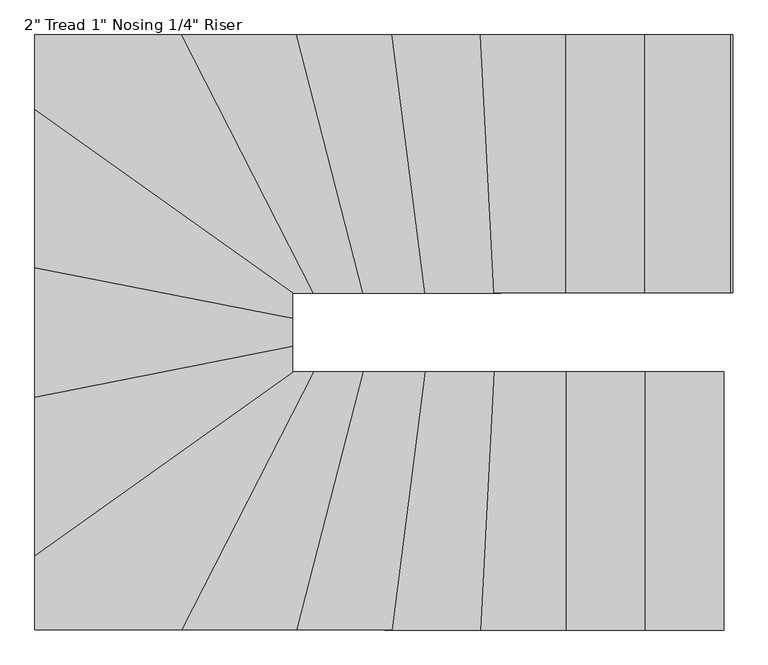
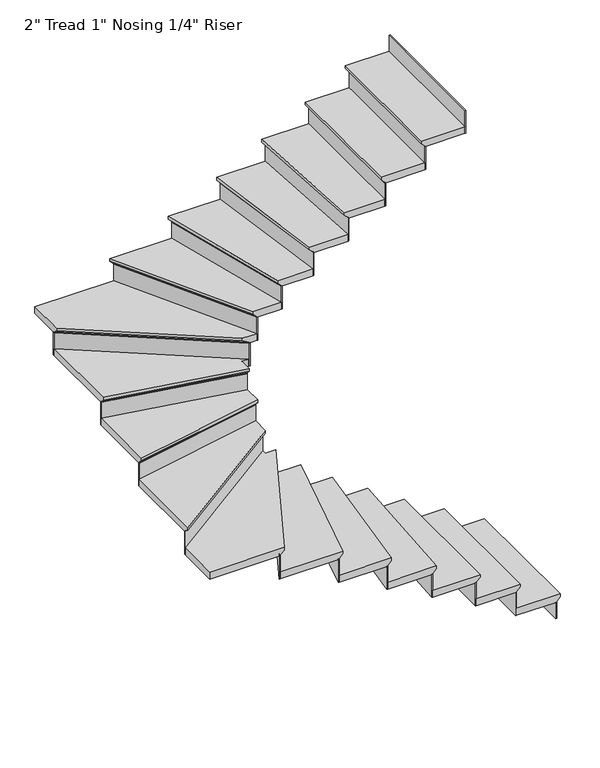
"""IFC4 building model written with IfcOpenShell, lengths in millimetres: stair flight geometry."""

from ifc_helpers import new_model, si_unit, origin, place, context, project, spatial, faceted_brep, source, transform, mapped, element, save


def stair_flight_5420025d(model_context):
    return source(origin(), model_context, "Body", "Brep", [
        faceted_brep([(-1761.7449167, -345.7070853, 3350.6833333), (-1761.7449167, -345.7070853, 3369.7333333), (-1761.7449167, -1260.1070853, 3369.7333333), (-1761.7449167, -1260.1070853, 3350.6833333), (-1787.1449167, -345.7070853, 3325.2833333), (-1787.1449167, -1260.1070853, 3325.2833333), (-2066.5449167, -345.7070853, 3369.7333333), (-2066.5449167, -1260.1070853, 3369.7333333), (-1787.1449167, -1260.1070853, 3318.9333333), (-2066.5449167, -1260.1070853, 3318.9333333), (-2066.5449167, -345.7070853, 3318.9333333), (-1787.1449167, -345.7070853, 3318.9333333)], [[[0, 1, 2, 3]], [[4, 0, 3, 5]], [[2, 1, 6, 7]], [[8, 9, 10, 11]], [[2, 7, 9, 8, 5, 3]], [[8, 11, 4, 5]], [[6, 1, 0, 4, 11, 10]], [[7, 6, 10, 9]]]),
        faceted_brep([(-1787.1449167, -345.7070853, 3318.9333333), (-1787.1449167, -345.7070853, 3200.4), (-1793.4949167, -345.7070853, 3200.4), (-1793.4949167, -345.7070853, 3318.9333333), (-1787.1449167, -1260.1070853, 3318.9333333), (-1793.4949167, -1260.1070853, 3318.9333333), (-1793.4949167, -1260.1070853, 3200.4), (-1787.1449167, -1260.1070853, 3200.4)], [[[0, 1, 2, 3]], [[4, 5, 6, 7]], [[1, 0, 4, 7]], [[2, 1, 7, 6]], [[3, 2, 6, 5]], [[0, 3, 5, 4]]]),
        faceted_brep([(-2066.5449167, -345.7070853, 3488.2666667), (-2066.5449167, -345.7070853, 3318.9333333), (-2072.8949167, -345.7070853, 3318.9333333), (-2072.8949167, -345.7070853, 3488.2666667), (-2066.5449167, -1260.1070853, 3488.2666667), (-2072.8949167, -1260.1070853, 3488.2666667), (-2072.8949167, -1260.1070853, 3318.9333333), (-2066.5449167, -1260.1070853, 3318.9333333)], [[[0, 1, 2, 3]], [[4, 5, 6, 7]], [[1, 0, 4, 7]], [[2, 1, 7, 6]], [[3, 2, 6, 5]], [[0, 3, 5, 4]]]),
        faceted_brep([(-2041.1449167, -1260.1070853, 3539.0666667), (-2041.1449167, -345.7070853, 3539.0666667), (-2345.9449167, -345.7070853, 3539.0666667), (-2345.9449167, -1260.1070853, 3539.0666667), (-2066.5449167, -1260.1070853, 3488.2666667), (-2345.9449167, -1260.1070853, 3488.2666667), (-2345.9449167, -345.7070853, 3488.2666667), (-2066.5449167, -345.7070853, 3488.2666667), (-2066.5449167, -1260.1070853, 3494.6166667), (-2041.1449167, -1260.1070853, 3520.0166667), (-2066.5449167, -345.7070853, 3494.6166667), (-2041.1449167, -345.7070853, 3520.0166667)], [[[0, 1, 2, 3]], [[4, 5, 6, 7]], [[0, 3, 5, 4, 8, 9]], [[4, 7, 10, 8]], [[2, 1, 11, 10, 7, 6]], [[3, 2, 6, 5]], [[11, 1, 0, 9]], [[10, 11, 9, 8]]]),
        faceted_brep([(-2345.9449167, -345.7070853, 3657.6), (-2345.9449167, -345.7070853, 3488.2666667), (-2352.2949167, -345.7070853, 3488.2666667), (-2352.2949167, -345.7070853, 3657.6), (-2345.9449167, -1260.1070853, 3657.6), (-2352.2949167, -1260.1070853, 3657.6), (-2352.2949167, -1260.1070853, 3488.2666667), (-2345.9449167, -1260.1070853, 3488.2666667)], [[[0, 1, 2, 3]], [[4, 5, 6, 7]], [[1, 0, 4, 7]], [[2, 1, 7, 6]], [[3, 2, 6, 5]], [[0, 3, 5, 4]]]),
        faceted_brep([(-2320.5449167, -1260.1070853, 3708.4), (-2320.5449167, -345.7070853, 3708.4), (-2601.6120781, -345.7070853, 3708.4), (-2649.1463485, -1260.1070853, 3708.4), (-2345.9449167, -1260.1070853, 3657.6), (-2649.1463485, -1260.1070853, 3657.6), (-2601.6120781, -345.7070853, 3657.6), (-2345.9449167, -345.7070853, 3657.6), (-2345.9449167, -1260.1070853, 3663.95), (-2320.5449167, -1260.1070853, 3689.35), (-2345.9449167, -345.7070853, 3663.95), (-2320.5449167, -345.7070853, 3689.35)], [[[0, 1, 2, 3]], [[4, 5, 6, 7]], [[0, 3, 5, 4, 8, 9]], [[4, 7, 10, 8]], [[2, 1, 11, 10, 7, 6]], [[3, 2, 6, 5]], [[11, 1, 0, 9]], [[10, 11, 9, 8]]]),
        faceted_brep([(-2601.6120781, -345.7070853, 3826.9333333), (-2601.6120781, -345.7070853, 3657.6), (-2607.9706523, -345.7070853, 3657.6), (-2607.9706523, -345.7070853, 3826.9333333), (-2649.1463485, -1260.1070853, 3826.9333333), (-2655.5049227, -1260.1070853, 3826.9333333), (-2655.5049227, -1260.1070853, 3657.6), (-2649.1463485, -1260.1070853, 3657.6)], [[[0, 1, 2, 3]], [[4, 5, 6, 7]], [[1, 0, 4, 7]], [[2, 1, 7, 6]], [[3, 2, 6, 5]], [[0, 3, 5, 4]]]),
        faceted_brep([(-2623.7120519, -1260.1070853, 3877.7333333), (-2576.1777815, -345.7070853, 3877.7333333), (-2845.778778, -345.7070853, 3877.7333333), (-2964.1348296, -1260.1070853, 3877.7333333), (-2649.1463485, -1260.1070853, 3826.9333333), (-2964.1348296, -1260.1070853, 3826.9333333), (-2845.778778, -345.7070853, 3826.9333333), (-2601.6120781, -345.7070853, 3826.9333333), (-2649.1463485, -1260.1070853, 3833.2833333), (-2623.7120519, -1260.1070853, 3858.6833333), (-2601.6120781, -345.7070853, 3833.2833333), (-2576.1777815, -345.7070853, 3858.6833333)], [[[0, 1, 2, 3]], [[4, 5, 6, 7]], [[0, 3, 5, 4, 8, 9]], [[4, 7, 10, 8]], [[2, 1, 11, 10, 7, 6]], [[3, 2, 6, 5]], [[11, 1, 0, 9]], [[10, 11, 9, 8]]]),
        faceted_brep([(-2845.778778, -345.7070853, 3996.2666667), (-2845.778778, -345.7070853, 3826.9333333), (-2852.1817497, -345.7070853, 3826.9333333), (-2852.1817497, -345.7070853, 3996.2666667), (-2964.1348296, -1260.1070853, 3996.2666667), (-2970.5378014, -1260.1070853, 3996.2666667), (-2970.5378014, -1260.1070853, 3826.9333333), (-2964.1348296, -1260.1070853, 3826.9333333)], [[[0, 1, 2, 3]], [[4, 5, 6, 7]], [[1, 0, 4, 7]], [[2, 1, 7, 6]], [[3, 2, 6, 5]], [[0, 3, 5, 4]]]),
        faceted_brep([(-2938.5229425, -1260.1070853, 4047.0666667), (-2820.1668908, -345.7070853, 4047.0666667), (-3067.4060004, -345.7070853, 4047.0666667), (-3302.5364478, -1260.1070853, 4047.0666667), (-2964.1348296, -1260.1070853, 3996.2666667), (-3302.5364478, -1260.1070853, 3996.2666667), (-3067.4060004, -345.7070853, 3996.2666667), (-2845.778778, -345.7070853, 3996.2666667), (-2964.1348296, -1260.1070853, 4002.6166667), (-2938.5229425, -1260.1070853, 4028.0166667), (-2845.778778, -345.7070853, 4002.6166667), (-2820.1668908, -345.7070853, 4028.0166667)], [[[0, 1, 2, 3]], [[4, 5, 6, 7]], [[0, 3, 5, 4, 8, 9]], [[4, 7, 10, 8]], [[2, 1, 11, 10, 7, 6]], [[3, 2, 6, 5]], [[11, 1, 0, 9]], [[10, 11, 9, 8]]]),
        faceted_brep([(-3067.4060004, -345.7070853, 4165.6), (-3067.4060004, -345.7070853, 3996.2666667), (-3073.9625773, -345.7070853, 3996.2666667), (-3073.9625773, -345.7070853, 4165.6), (-3302.5364478, -1260.1070853, 4165.6), (-3309.0930247, -1260.1070853, 4165.6), (-3309.0930247, -1260.1070853, 3996.2666667), (-3302.5364478, -1260.1070853, 3996.2666667)], [[[0, 1, 2, 3]], [[4, 5, 6, 7]], [[1, 0, 4, 7]], [[2, 1, 7, 6]], [[3, 2, 6, 5]], [[0, 3, 5, 4]]]),
        faceted_brep([(-3276.3101404, -1260.1070853, 4216.4), (-3041.179693, -345.7070853, 4216.4), (-3243.7526365, -345.7070853, 4216.4), (-3712.5772578, -1260.1070853, 4216.4), (-3302.5364478, -1260.1070853, 4165.6), (-3712.5772578, -1260.1070853, 4165.6), (-3243.7526365, -345.7070853, 4165.6), (-3067.4060004, -345.7070853, 4165.6), (-3302.5364478, -1260.1070853, 4171.95), (-3276.3101404, -1260.1070853, 4197.35), (-3067.4060004, -345.7070853, 4171.95), (-3041.179693, -345.7070853, 4197.35)], [[[0, 1, 2, 3]], [[4, 5, 6, 7]], [[0, 3, 5, 4, 8, 9]], [[4, 7, 10, 8]], [[2, 1, 11, 10, 7, 6]], [[3, 2, 6, 5]], [[11, 1, 0, 9]], [[10, 11, 9, 8]]]),
        faceted_brep([(-3243.7526365, -345.7070853, 4334.9333333), (-3243.7526365, -345.7070853, 4165.6), (-3250.8886197, -345.7070853, 4165.6), (-3250.8886197, -345.7070853, 4334.9333333), (-3712.5772578, -1260.1070853, 4334.9333333), (-3719.713241, -1260.1070853, 4334.9333333), (-3719.713241, -1260.1070853, 4165.6), (-3712.5772578, -1260.1070853, 4165.6)], [[[0, 1, 2, 3]], [[4, 5, 6, 7]], [[1, 0, 4, 7]], [[2, 1, 7, 6]], [[3, 2, 6, 5]], [[0, 3, 5, 4]]]),
        faceted_brep([(-4203.8766085, -966.4259516, 4385.7333333), (-4203.8766085, -1260.1070853, 4385.7333333), (-3684.0333253, -1260.1070853, 4385.7333333), (-3215.208704, -345.7070853, 4385.7333333), (-3289.4766085, -345.7070853, 4385.7333333), (-3289.4766085, -316.1520025, 4385.7333333), (-4203.8766085, -1260.1070853, 4334.9333333), (-4203.8766085, -966.4259516, 4334.9333333), (-3289.4766085, -316.1520025, 4334.9333333), (-3289.4766085, -345.7070853, 4334.9333333), (-3243.7526365, -345.7070853, 4334.9333333), (-3712.5772578, -1260.1070853, 4334.9333333), (-3712.5772578, -1260.1070853, 4341.2833333), (-3684.0333253, -1260.1070853, 4366.6833333), (-3243.7526365, -345.7070853, 4341.2833333), (-3215.208704, -345.7070853, 4366.6833333)], [[[0, 1, 2, 3, 4, 5]], [[6, 7, 8, 9, 10, 11]], [[1, 0, 7, 6]], [[2, 1, 6, 11, 12, 13]], [[11, 10, 14, 12]], [[4, 3, 15, 14, 10, 9]], [[5, 4, 9, 8]], [[0, 5, 8, 7]], [[15, 3, 2, 13]], [[14, 15, 13, 12]]]),
        faceted_brep([(-3289.4766085, -316.1520025, 4504.2666667), (-3289.4766085, -316.1520025, 4334.9333333), (-3289.4766085, -308.3600277, 4334.9333333), (-3289.4766085, -308.3600277, 4504.2666667), (-4203.8766085, -966.4259516, 4504.2666667), (-4203.8766085, -958.6339768, 4504.2666667), (-4203.8766085, -958.6339768, 4334.9333333), (-4203.8766085, -966.4259516, 4334.9333333)], [[[0, 1, 2, 3]], [[4, 5, 6, 7]], [[1, 0, 4, 7]], [[2, 1, 7, 6]], [[3, 2, 6, 5]], [[0, 3, 5, 4]]]),
        faceted_brep([(-4203.8766085, -997.5938508, 4555.0666667), (-3289.4766085, -347.3199017, 4555.0666667), (-3289.4766085, -229.6979154, 4555.0666667), (-4203.8766085, -409.9387717, 4555.0666667), (-4203.8766085, -966.4259516, 4504.2666667), (-4203.8766085, -409.9387717, 4504.2666667), (-3289.4766085, -229.6979154, 4504.2666667), (-3289.4766085, -316.1520025, 4504.2666667), (-4203.8766085, -966.4259516, 4510.6166667), (-4203.8766085, -997.5938508, 4536.0166667), (-3289.4766085, -316.1520025, 4510.6166667), (-3289.4766085, -347.3199017, 4536.0166667)], [[[0, 1, 2, 3]], [[4, 5, 6, 7]], [[0, 3, 5, 4, 8, 9]], [[4, 7, 10, 8]], [[2, 1, 11, 10, 7, 6]], [[3, 2, 6, 5]], [[11, 1, 0, 9]], [[10, 11, 9, 8]]]),
        faceted_brep([(-3289.4766085, -229.6979154, 4673.6), (-3289.4766085, -229.6979154, 4504.2666667), (-3289.4766085, -223.22573, 4504.2666667), (-3289.4766085, -223.22573, 4673.6), (-4203.8766085, -409.9387717, 4673.6), (-4203.8766085, -403.4665863, 4673.6), (-4203.8766085, -403.4665863, 4504.2666667), (-4203.8766085, -409.9387717, 4504.2666667)], [[[0, 1, 2, 3]], [[4, 5, 6, 7]], [[1, 0, 4, 7]], [[2, 1, 7, 6]], [[3, 2, 6, 5]], [[0, 3, 5, 4]]]),
        faceted_brep([(-4203.8766085, -435.8275135, 4724.4), (-3289.4766085, -255.5866572, 4724.4), (-3289.4766085, -130.5387717, 4724.4), (-4203.8766085, 49.7020846, 4724.4), (-4203.8766085, -409.9387717, 4673.6), (-4203.8766085, 49.7020846, 4673.6), (-3289.4766085, -130.5387717, 4673.6), (-3289.4766085, -229.6979154, 4673.6), (-4203.8766085, -409.9387717, 4679.95), (-4203.8766085, -435.8275135, 4705.35), (-3289.4766085, -229.6979154, 4679.95), (-3289.4766085, -255.5866572, 4705.35)], [[[0, 1, 2, 3]], [[4, 5, 6, 7]], [[0, 3, 5, 4, 8, 9]], [[4, 7, 10, 8]], [[2, 1, 11, 10, 7, 6]], [[3, 2, 6, 5]], [[11, 1, 0, 9]], [[10, 11, 9, 8]]]),
        faceted_brep([(-3289.4766085, -130.5387717, 4842.9333333), (-3289.4766085, -130.5387717, 4673.6), (-3289.4766085, -124.0665863, 4673.6), (-3289.4766085, -124.0665863, 4842.9333333), (-4203.8766085, 49.7020846, 4842.9333333), (-4203.8766085, 56.17427, 4842.9333333), (-4203.8766085, 56.17427, 4673.6), (-4203.8766085, 49.7020846, 4673.6)], [[[0, 1, 2, 3]], [[4, 5, 6, 7]], [[1, 0, 4, 7]], [[2, 1, 7, 6]], [[3, 2, 6, 5]], [[0, 3, 5, 4]]]),
        faceted_brep([(-4203.8766085, 23.8133428, 4893.7333333), (-3289.4766085, -156.4275135, 4893.7333333), (-3289.4766085, -66.3070853, 4893.7333333), (-3243.381134, -66.3070853, 4893.7333333), (-4203.8766085, 616.7475793, 4893.7333333), (-4203.8766085, 49.7020846, 4842.9333333), (-4203.8766085, 616.7475793, 4842.9333333), (-3243.381134, -66.3070853, 4842.9333333), (-3289.4766085, -66.3070853, 4842.9333333), (-3289.4766085, -130.5387717, 4842.9333333), (-4203.8766085, 49.7020846, 4849.2833333), (-4203.8766085, 23.8133428, 4874.6833333), (-3289.4766085, -130.5387717, 4849.2833333), (-3289.4766085, -156.4275135, 4874.6833333)], [[[0, 1, 2, 3, 4]], [[5, 6, 7, 8, 9]], [[0, 4, 6, 5, 10, 11]], [[5, 9, 12, 10]], [[2, 1, 13, 12, 9, 8]], [[3, 2, 8, 7]], [[4, 3, 7, 6]], [[13, 1, 0, 11]], [[12, 13, 11, 10]]]),
        faceted_brep([(-3243.381134, -66.3070853, 5012.2666667), (-3243.381134, -66.3070853, 4842.9333333), (-3232.4242415, -66.3070853, 4842.9333333), (-3232.4242415, -66.3070853, 5012.2666667), (-4203.8766085, 616.7475793, 5012.2666667), (-4203.8766085, 624.5395541, 5012.2666667), (-4203.8766085, 624.5395541, 4842.9333333), (-4203.8766085, 616.7475793, 4842.9333333)], [[[0, 1, 2, 3]], [[4, 5, 6, 7]], [[1, 0, 4, 7]], [[2, 1, 7, 6]], [[3, 2, 6, 5]], [[0, 3, 5, 4]]]),
        faceted_brep([(-3655.4893928, 848.0929147, 5063.0666667), (-4203.8766085, 848.0929147, 5063.0666667), (-4203.8766085, 585.5796802, 5063.0666667), (-3287.208704, -66.3070853, 5063.0666667), (-3186.6647715, -66.3070853, 5063.0666667), (-4203.8766085, 848.0929147, 5012.2666667), (-3655.4893928, 848.0929147, 5012.2666667), (-3186.6647715, -66.3070853, 5012.2666667), (-3243.381134, -66.3070853, 5012.2666667), (-4203.8766085, 616.7475793, 5012.2666667), (-4203.8766085, 616.7475793, 5018.6166667), (-4203.8766085, 585.5796802, 5044.0166667), (-3243.381134, -66.3070853, 5018.6166667), (-3287.208704, -66.3070853, 5044.0166667)], [[[0, 1, 2, 3, 4]], [[5, 6, 7, 8, 9]], [[1, 0, 6, 5]], [[2, 1, 5, 9, 10, 11]], [[9, 8, 12, 10]], [[4, 3, 13, 12, 8, 7]], [[0, 4, 7, 6]], [[13, 3, 2, 11]], [[12, 13, 11, 10]]]),
        faceted_brep([(-3186.6647715, -66.3070853, 5181.6), (-3186.6647715, -66.3070853, 5012.2666667), (-3179.5287883, -66.3070853, 5012.2666667), (-3179.5287883, -66.3070853, 5181.6), (-3655.4893928, 848.0929147, 5181.6), (-3648.3534096, 848.0929147, 5181.6), (-3648.3534096, 848.0929147, 5012.2666667), (-3655.4893928, 848.0929147, 5012.2666667)], [[[0, 1, 2, 3]], [[4, 5, 6, 7]], [[1, 0, 4, 7]], [[2, 1, 7, 6]], [[3, 2, 6, 5]], [[0, 3, 5, 4]]]),
        faceted_brep([(-3684.0333253, 848.0929147, 5232.4), (-3215.208704, -66.3070853, 5232.4), (-3014.9533855, -66.3070853, 5232.4), (-3250.0838329, 848.0929147, 5232.4), (-3655.4893928, 848.0929147, 5181.6), (-3250.0838329, 848.0929147, 5181.6), (-3014.9533855, -66.3070853, 5181.6), (-3186.6647715, -66.3070853, 5181.6), (-3655.4893928, 848.0929147, 5187.95), (-3684.0333253, 848.0929147, 5213.35), (-3186.6647715, -66.3070853, 5187.95), (-3215.208704, -66.3070853, 5213.35)], [[[0, 1, 2, 3]], [[4, 5, 6, 7]], [[0, 3, 5, 4, 8, 9]], [[4, 7, 10, 8]], [[2, 1, 11, 10, 7, 6]], [[3, 2, 6, 5]], [[11, 1, 0, 9]], [[10, 11, 9, 8]]]),
        faceted_brep([(-3014.9533855, -66.3070853, 5350.9333333), (-3014.9533855, -66.3070853, 5181.6), (-3008.3968086, -66.3070853, 5181.6), (-3008.3968086, -66.3070853, 5350.9333333), (-3250.0838329, 848.0929147, 5350.9333333), (-3243.5272561, 848.0929147, 5350.9333333), (-3243.5272561, 848.0929147, 5181.6), (-3250.0838329, 848.0929147, 5181.6)], [[[0, 1, 2, 3]], [[4, 5, 6, 7]], [[1, 0, 4, 7]], [[2, 1, 7, 6]], [[3, 2, 6, 5]], [[0, 3, 5, 4]]]),
        faceted_brep([(-3276.3101404, 848.0929147, 5401.7333333), (-3041.179693, -66.3070853, 5401.7333333), (-2794.5550037, -66.3070853, 5401.7333333), (-2912.9110554, 848.0929147, 5401.7333333), (-3250.0838329, 848.0929147, 5350.9333333), (-2912.9110554, 848.0929147, 5350.9333333), (-2794.5550037, -66.3070853, 5350.9333333), (-3014.9533855, -66.3070853, 5350.9333333), (-3250.0838329, 848.0929147, 5357.2833333), (-3276.3101404, 848.0929147, 5382.6833333), (-3014.9533855, -66.3070853, 5357.2833333), (-3041.179693, -66.3070853, 5382.6833333)], [[[0, 1, 2, 3]], [[4, 5, 6, 7]], [[0, 3, 5, 4, 8, 9]], [[4, 7, 10, 8]], [[2, 1, 11, 10, 7, 6]], [[3, 2, 6, 5]], [[11, 1, 0, 9]], [[10, 11, 9, 8]]]),
        faceted_brep([(-2794.5550037, -66.3070853, 5520.2666667), (-2794.5550037, -66.3070853, 5350.9333333), (-2788.152032, -66.3070853, 5350.9333333), (-2788.152032, -66.3070853, 5520.2666667), (-2912.9110554, 848.0929147, 5520.2666667), (-2906.5080836, 848.0929147, 5520.2666667), (-2906.5080836, 848.0929147, 5350.9333333), (-2912.9110554, 848.0929147, 5350.9333333)], [[[0, 1, 2, 3]], [[4, 5, 6, 7]], [[1, 0, 4, 7]], [[2, 1, 7, 6]], [[3, 2, 6, 5]], [[0, 3, 5, 4]]]),
        faceted_brep([(-2938.5229425, 848.0929147, 5571.0666667), (-2820.1668908, -66.3070853, 5571.0666667), (-2550.7434848, -66.3070853, 5571.0666667), (-2598.2777552, 848.0929147, 5571.0666667), (-2912.9110554, 848.0929147, 5520.2666667), (-2598.2777552, 848.0929147, 5520.2666667), (-2550.7434848, -66.3070853, 5520.2666667), (-2794.5550037, -66.3070853, 5520.2666667), (-2912.9110554, 848.0929147, 5526.6166667), (-2938.5229425, 848.0929147, 5552.0166667), (-2794.5550037, -66.3070853, 5526.6166667), (-2820.1668908, -66.3070853, 5552.0166667)], [[[0, 1, 2, 3]], [[4, 5, 6, 7]], [[0, 3, 5, 4, 8, 9]], [[4, 7, 10, 8]], [[2, 1, 11, 10, 7, 6]], [[3, 2, 6, 5]], [[11, 1, 0, 9]], [[10, 11, 9, 8]]]),
        faceted_brep([(-2550.7434848, -66.3070853, 5689.6), (-2550.7434848, -66.3070853, 5520.2666667), (-2544.3849106, -66.3070853, 5520.2666667), (-2544.3849106, -66.3070853, 5689.6), (-2598.2777552, 848.0929147, 5689.6), (-2591.9191811, 848.0929147, 5689.6), (-2591.9191811, 848.0929147, 5520.2666667), (-2598.2777552, 848.0929147, 5520.2666667)], [[[0, 1, 2, 3]], [[4, 5, 6, 7]], [[1, 0, 4, 7]], [[2, 1, 7, 6]], [[3, 2, 6, 5]], [[0, 3, 5, 4]]]),
        faceted_brep([(-2623.7120519, 848.0929147, 5740.4), (-2576.1777815, -66.3070853, 5740.4), (-2295.1449167, -66.3070853, 5740.4), (-2295.1449167, 848.0929147, 5740.4), (-2598.2777552, 848.0929147, 5689.6), (-2295.1449167, 848.0929147, 5689.6), (-2295.1449167, -66.3070853, 5689.6), (-2550.7434848, -66.3070853, 5689.6), (-2598.2777552, 848.0929147, 5695.95), (-2623.7120519, 848.0929147, 5721.35), (-2550.7434848, -66.3070853, 5695.95), (-2576.1777815, -66.3070853, 5721.35)], [[[0, 1, 2, 3]], [[4, 5, 6, 7]], [[0, 3, 5, 4, 8, 9]], [[4, 7, 10, 8]], [[2, 1, 11, 10, 7, 6]], [[3, 2, 6, 5]], [[11, 1, 0, 9]], [[10, 11, 9, 8]]]),
        faceted_brep([(-2295.1449167, -66.3070853, 5858.9333333), (-2295.1449167, -66.3070853, 5689.6), (-2288.7949167, -66.3070853, 5689.6), (-2288.7949167, -66.3070853, 5858.9333333), (-2295.1449167, 848.0929147, 5858.9333333), (-2288.7949167, 848.0929147, 5858.9333333), (-2288.7949167, 848.0929147, 5689.6), (-2295.1449167, 848.0929147, 5689.6)], [[[0, 1, 2, 3]], [[4, 5, 6, 7]], [[1, 0, 4, 7]], [[2, 1, 7, 6]], [[3, 2, 6, 5]], [[0, 3, 5, 4]]]),
        faceted_brep([(-2320.5449167, 848.0929147, 5909.7333333), (-2320.5449167, -66.3070853, 5909.7333333), (-2015.7449167, -66.3070853, 5909.7333333), (-2015.7449167, 848.0929147, 5909.7333333), (-2295.1449167, 848.0929147, 5858.9333333), (-2015.7449167, 848.0929147, 5858.9333333), (-2015.7449167, -66.3070853, 5858.9333333), (-2295.1449167, -66.3070853, 5858.9333333), (-2295.1449167, 848.0929147, 5865.2833333), (-2320.5449167, 848.0929147, 5890.6833333), (-2295.1449167, -66.3070853, 5865.2833333), (-2320.5449167, -66.3070853, 5890.6833333)], [[[0, 1, 2, 3]], [[4, 5, 6, 7]], [[0, 3, 5, 4, 8, 9]], [[4, 7, 10, 8]], [[2, 1, 11, 10, 7, 6]], [[3, 2, 6, 5]], [[11, 1, 0, 9]], [[10, 11, 9, 8]]]),
        faceted_brep([(-2015.7449167, -66.3070853, 6028.2666667), (-2015.7449167, -66.3070853, 5858.9333333), (-2009.3949167, -66.3070853, 5858.9333333), (-2009.3949167, -66.3070853, 6028.2666667), (-2015.7449167, 848.0929147, 6028.2666667), (-2009.3949167, 848.0929147, 6028.2666667), (-2009.3949167, 848.0929147, 5858.9333333), (-2015.7449167, 848.0929147, 5858.9333333)], [[[0, 1, 2, 3]], [[4, 5, 6, 7]], [[1, 0, 4, 7]], [[2, 1, 7, 6]], [[3, 2, 6, 5]], [[0, 3, 5, 4]]]),
        faceted_brep([(-1736.3449167, -66.3070853, 6197.6), (-1736.3449167, -66.3070853, 6028.2666667), (-1729.9949167, -66.3070853, 6028.2666667), (-1729.9949167, -66.3070853, 6197.6), (-1736.3449167, 848.0929147, 6197.6), (-1729.9949167, 848.0929147, 6197.6), (-1729.9949167, 848.0929147, 6028.2666667), (-1736.3449167, 848.0929147, 6028.2666667)], [[[0, 1, 2, 3]], [[4, 5, 6, 7]], [[1, 0, 4, 7]], [[2, 1, 7, 6]], [[3, 2, 6, 5]], [[0, 3, 5, 4]]]),
        faceted_brep([(-2041.1449167, 848.0929147, 6079.0666667), (-2041.1449167, -66.3070853, 6079.0666667), (-1736.3449167, -66.3070853, 6079.0666667), (-1736.3449167, 848.0929147, 6079.0666667), (-2015.7449167, 848.0929147, 6028.2666667), (-1736.3449167, 848.0929147, 6028.2666667), (-1736.3449167, -66.3070853, 6028.2666667), (-2015.7449167, -66.3070853, 6028.2666667), (-2015.7449167, 848.0929147, 6034.6166667), (-2041.1449167, 848.0929147, 6060.0166667), (-2015.7449167, -66.3070853, 6034.6166667), (-2041.1449167, -66.3070853, 6060.0166667)], [[[0, 1, 2, 3]], [[4, 5, 6, 7]], [[0, 3, 5, 4, 8, 9]], [[4, 7, 10, 8]], [[2, 1, 11, 10, 7, 6]], [[3, 2, 6, 5]], [[11, 1, 0, 9]], [[10, 11, 9, 8]]]),
    ])


if __name__ == "__main__":
    model = new_model("IFC4")
    model_context = context("Model", 3, world=origin())
    ifc_project = project(units=[si_unit("LENGTHUNIT", "METRE", prefix="MILLI")], contexts=[model_context])
    site = spatial("IfcSite", under=ifc_project)
    building = spatial("IfcBuilding", under=site)
    placement = place(None, origin())
    stair_flight_shape = stair_flight_5420025d(model_context)
    element("IfcStairFlight", 1, ObjectType="2\" Tread 1\" Nosing 1/4\" Riser", at=placement, inside=building, context=model_context, shape_type="MappedRepresentation", body=[
        mapped(stair_flight_shape, transform((0.0, 0.0, 0.0), x_axis=(1.0, 0.0, 0.0), y_axis=(0.0, 1.0, 0.0), z_axis=(0.0, 0.0, 1.0))),
    ])
    save(model, "model.ifc")
